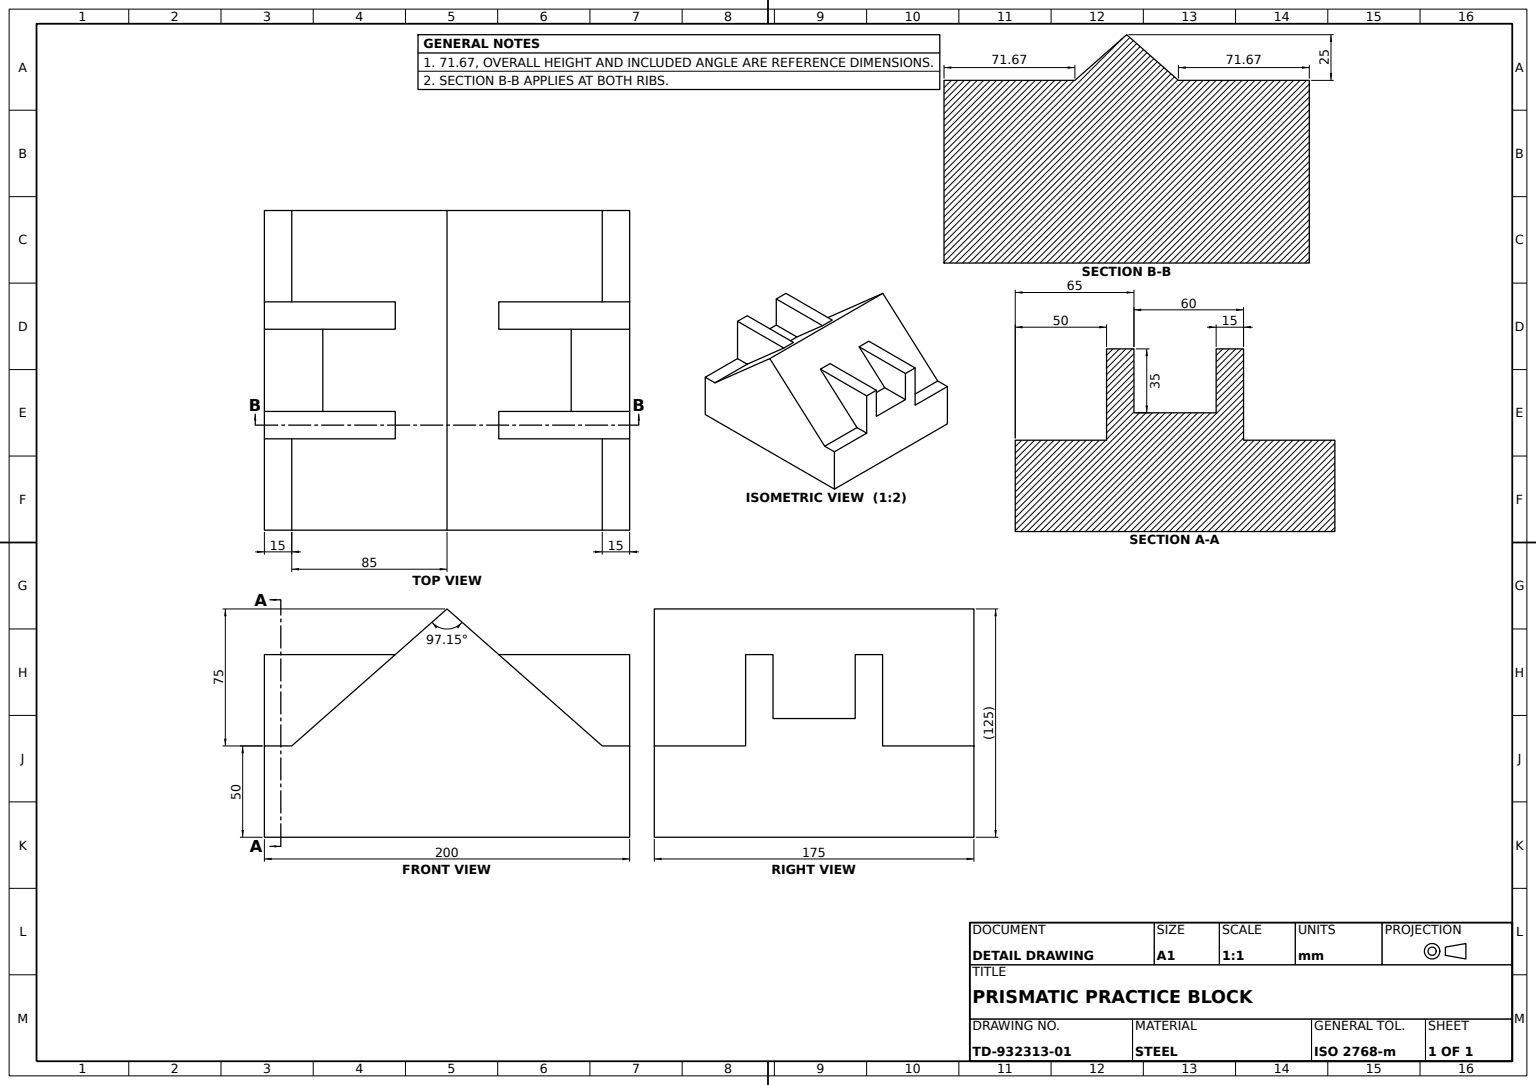
SolidWorks part; units mm, degrees
material "Plain Carbon Steel"
ref_plane "Front Plane" through (0, 0, 0) normal (0, 0, 1) x (1, 0, 0)
ref_plane "Top Plane" through (0, 0, 0) normal (0, 1, 0) x (1, 0, 0)
ref_plane "Right Plane" through (0, 0, 0) normal (1, 0, 0) x (0, 0, -1)
sketch "Base Block Profile" plane through (0, 0, 0) normal (0, 0, 1) x (1, 0, 0)
  line L0 (0, 0) -> (200, 0)
  line L1 (200, 0) -> (200, 175)
  line L2 (0, 0) -> (0, 175)
  line L3 (0, 175) -> (200, 175)
  dimension "D1" = 200
  dimension "D2" = 175
extrude "Base Block" add sketch "Base Block Profile" against normal blind 50
sketch "Notched Boss Profile 175" plane through (0, 0, 0) normal (0, -1, 0) x (1, 0, 0)
  line L0 (0, -50) -> (200, -50) construction
  line L3 (0, 0) -> (200, 0) construction
  line L4 (15, 0) -> (100, 75)
  line L6 (100, 75) -> (185, 0)
  line L7 (15, 0) -> (185, 0)
  line L11 (200, 0) -> (0, 0)
  line L12 (0, 0) -> (0, -50)
  line L13 (0, -50) -> (200, -50)
  line L14 (200, -50) -> (200, 0)
  line L16 (0, 0) -> (0, -50)
  line L17 (0, -50) -> (200, -50)
  line L18 (200, -50) -> (200, 0)
  line M6 (200, 0) -> (0, 0)
  dimension "D1" = 75
  dimension "D2" = 15
  dimension "D3" = 15
  dimension "D4" = 125
  dimension "D5" = 85
  dimension "D6" = 0
extrude "Notched Boss 175" add sketch "Notched Boss Profile 175" against normal blind 175 contours L6 L4 M6
sketch "Notched Boss Profile 200" plane through (200, 0, 0) normal (1, 0, 0) x (0, 0, -1)
  line L0 (0, 125) -> (0, 50)
  line L1 (0, 0) -> (0, 175) construction
  line L2 (0, 50) -> (-50, 50)
  line L4 (-50, 50) -> (-50, 65)
  line L5 (-50, 65) -> (-15, 65)
  line L6 (-75, 0) -> (0, 0) construction
  line L7 (0, 125) -> (-50, 125)
  line L8 (-50, 125) -> (-50, 110)
  line L9 (-50, 110) -> (-15, 110)
  line L10 (0, 50) -> (-15, 50)
  line L11 (-15, 65) -> (-15, 110)
  line M9 (0, 175) -> (0, 0)
  dimension "D1" = 50
  dimension "D2" = 15
  dimension "D3" = 60
  dimension "D4" = 15
  dimension "D5" = 15
  dimension "D6" = 35
  dimension "D7" = 50
  dimension "D8" = 65
extrude "Notched Boss 200" add sketch "Notched Boss Profile 200" against normal blind 200 contours L11 L5 L4 L2 L7 L8 L9 M9
